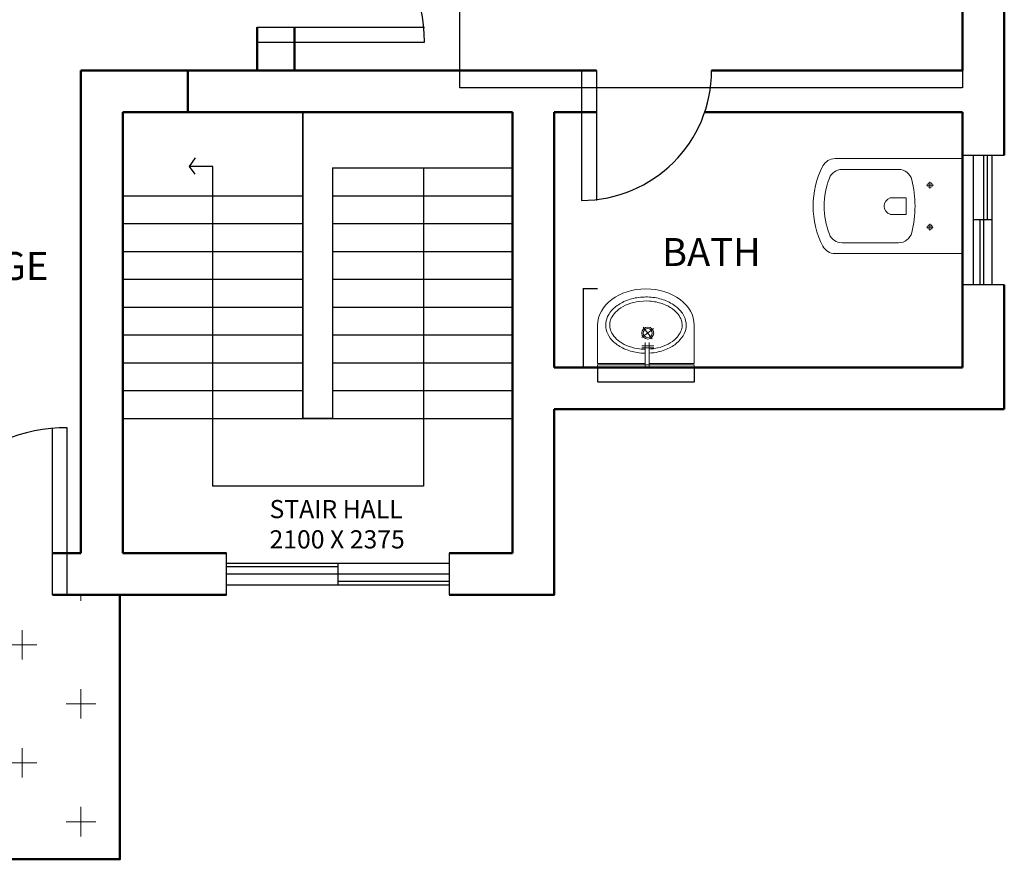
# Model space of a CAD drawing. Units: millimetres. Extents: x -857 to 54106, y -13666 to 13947.
# Tile 21 of 41: x 28540 to 33845, y 3904 to 8428. Entities that reach past the tile are written whole.
import ezdxf

# ---------------------------------------------------------------- set-up
doc = ezdxf.new("R2010")
doc.units = ezdxf.units.MM
for name, color, linetype, lineweight in [('A-ANNO-DIMS', 2, 'Continuous', 18), ('A-AREA-IDEN', 3, 'Continuous', 18), ('A-DOOR', 1, 'Continuous', 25), ('A-FLOR-FIXT', 8, 'Continuous', 18), ('A-FLOR-PATT', 252, 'Continuous', 13), ('A-FLOR-STRS', 30, 'Continuous', 25), ('A-GLAZ', 4, 'Continuous', 25), ('A-SANITARY FITTINGS', 25, 'Continuous', 15), ('A-WALL', 7, 'Continuous', 50)]:
    doc.layers.add(name, color=color, linetype=linetype, lineweight=lineweight)
doc.styles.get("Standard").update_dxf_attribs({"font": 'arial.ttf'})
doc.dimstyles.new('ISO-25', dxfattribs={"dimtxt": 2.5, "dimasz": 2.5, "dimexe": 1.25, "dimexo": 0.625, "dimtad": 1, "dimtxsty": 'Standard', "dimcen": 2.5, "dimadec": 0, "dimazin": 0, "dimtfac": 1, "dimtmove": 0, "dimatfit": 3, "dimfxl": 1, "dimarcsym": 0})

# ---------------------------------------------------------------- blocks, each defined once
blk = doc.blocks.new('A$C0124305E')
at = {"layer": 'A-SANITARY FITTINGS'}
for p, q in [((-8.42, 16.01), (-0.8, 16.01)), ((-0.8, 7.08), (-0.8, 16.01)), ((-7.73, 7.95), (-5.93, 5.62)), ((-4.31, 5.61), (-4.31, 7.96)), ((-3.91, 5.61), (-3.91, 7.96)), ((-5.66, 7.68), (-8, 5.88)), ((0, 7.08), (-4.99, 7.08)), ((0, 6.28), (-4.99, 6.28)), ((-0.8, -3.19), (-0.8, 6.28)), ((-8.42, -3.19), (-0.8, -3.19))]:
    blk.add_line(p, q, dxfattribs=at)
blk.add_lwpolyline([(-0.5, 16.01), (0, 16.01), (0, -3.19), (-0.5, -3.19)], close=True, dxfattribs=at)
for radius in [1.18, 0.885]:
    blk.add_circle((-6.83, 6.78), radius, dxfattribs=at)
at = {"layer": 'A-SANITARY FITTINGS', "extrusion": (0, 0, -1)}
blk.add_ellipse((-8.42, 6.41), major_axis=(0, 9.6), ratio=0.75, start_param=3.141593, end_param=6.283185, dxfattribs=at)
at = {"layer": 'A-SANITARY FITTINGS'}
for points, knots in [([(-2.82, 6.28), (-2.82, 5.74), (-2.87, 5.2), (-3.1, 3.74), (-3.37, 2.86), (-4.09, 1.28), (-4.55, 0.6), (-5.56, -0.5), (-6.12, -0.92), (-7.25, -1.45), (-7.83, -1.58), (-8.98, -1.59), (-9.55, -1.46), (-10.69, -0.93), (-11.25, -0.52), (-12.27, 0.57), (-12.72, 1.25), (-13.45, 2.82), (-13.72, 3.71), (-14.02, 5.56), (-14.05, 6.52), (-13.88, 8.41), (-13.67, 9.32), (-13.04, 10.99), (-12.62, 11.73), (-11.66, 12.96), (-11.12, 13.45), (-10, 14.13), (-9.43, 14.32), (-8.28, 14.45), (-7.7, 14.39), (-6.56, 14), (-5.99, 13.66), (-4.93, 12.71), (-4.44, 12.09), (-3.62, 10.62), (-3.3, 9.78), (-2.96, 8.29), (-2.87, 7.69), (-2.84, 7.08)], [1.58652, 1.58652, 1.58652, 1.58652, 1.780321, 1.780321, 2.120053, 2.120053, 2.459785, 2.459785, 2.799517, 2.799517, 3.139249, 3.139249, 3.478981, 3.478981, 3.818713, 3.818713, 4.158445, 4.158445, 4.498177, 4.498177, 4.837909, 4.837909, 5.177641, 5.177641, 5.517373, 5.517373, 5.857105, 5.857105, 6.196837, 6.196837, 6.536569, 6.536569, 6.876301, 6.876301, 7.216033, 7.216033, 7.555765, 7.555765, 7.774364, 7.774364, 7.774364, 7.774364]), ([(-3.62, 6.29), (-3.62, 5.76), (-3.67, 5.23), (-3.88, 3.96), (-4.1, 3.23), (-4.65, 1.95), (-4.98, 1.39), (-5.72, 0.46), (-6.12, 0.1), (-6.92, -0.44), (-7.32, -0.61), (-8.11, -0.8), (-8.5, -0.81), (-9.28, -0.69), (-9.68, -0.55), (-10.48, -0.08), (-10.89, 0.24), (-11.67, 1.13), (-12.05, 1.7), (-12.66, 3.01), (-12.9, 3.76), (-13.2, 5.38), (-13.25, 6.28), (-13.13, 8.02), (-12.95, 8.88), (-12.42, 10.42), (-12.06, 11.12), (-11.23, 12.25), (-10.77, 12.7), (-9.92, 13.26), (-9.53, 13.43), (-8.78, 13.62), (-8.41, 13.64), (-7.66, 13.54), (-7.28, 13.42), (-6.51, 13.02), (-6.12, 12.73), (-5.35, 11.95), (-4.97, 11.43), (-4.34, 10.23), (-4.08, 9.54), (-3.76, 8.24), (-3.67, 7.64), (-3.63, 7.03)], [1.58652, 1.58652, 1.58652, 1.58652, 1.790653, 1.790653, 2.093007, 2.093007, 2.384527, 2.384527, 2.676047, 2.676047, 2.967567, 2.967567, 3.259087, 3.259087, 3.550608, 3.550608, 3.842128, 3.842128, 4.155456, 4.155456, 4.468784, 4.468784, 4.806699, 4.806699, 5.144614, 5.144614, 5.482529, 5.482529, 5.820444, 5.820444, 6.099515, 6.099515, 6.378586, 6.378586, 6.657656, 6.657656, 6.936727, 6.936727, 7.23864, 7.23864, 7.540552, 7.540552, 7.774364, 7.774364, 7.774364, 7.774364])]:
    blk.add_open_spline(points, degree=3, knots=knots, dxfattribs=at)
blk = doc.blocks.new('A$C7d9d00ca')
at = {"layer": 'A-SANITARY FITTINGS'}
for p, q in [((0, 0), (-13.78, 0)), ((-13.78, -18.49), (-13.78, 0)), ((0, -18.49), (0, 0)), ((-9.94, -4.23), (-9.94, -5.23)), ((-3.84, -4.24), (-3.84, -5.24)), ((-10.42, -4.72), (-9.43, -4.72)), ((-3.36, -4.73), (-4.34, -4.73)), ((-12.2, -9.27), (-12.2, -17.48)), ((-1.57, -9.27), (-1.57, -17.48))]:
    blk.add_line(p, q, dxfattribs=at)
for points in [[(-8.08, -8.19), (-5.7, -8.19), (-5.7, -8.19), (-5.7, -10.48)], [(-8.08, -8.19), (-8.08, -10.48)]]:
    blk.add_lwpolyline(points, dxfattribs=at)
for centre in [(-9.94, -4.72), (-3.84, -4.73)]:
    blk.add_circle(centre, 0.342, dxfattribs=at)
for centre, radius, start, end in [((-6.89, -22.82), 15.93, 76.135, 103.8652), ((-10.24, -9.27), 1.97, 103.8652, 180), ((-3.54, -9.27), 1.97, 0.0003, 76.135), ((-6.89, -10.13), 1.24, 196.5098, 343.4902), ((-11.81, -18.49), 1.97, 180, 242.8074), ((-10.24, -17.48), 1.97, 180, 248.6555), ((-3.54, -17.48), 1.97, 291.3447, 0.0003), ((-1.97, -18.49), 1.97, 297.1926, 0), ((-6.89, -8.92), 11.16, 248.6555, 291.3447), ((-6.89, -8.92), 12.74, 242.8074, 297.1926)]:
    blk.add_arc(centre, radius, start, end, dxfattribs=at)
blk = doc.blocks.new('DOOR-900')
blk.add_line((11417.3, 9811.5), (12317.3, 9811.5))
blk.add_arc((11417.3, 9811.5), 900, 0, 90)
blk = doc.blocks.new('DOOR-700')
blk.add_line((8245.5, 10779.2), (8245.5, 11479.2))
blk.add_arc((8245.5, 10779.2), 700, 90, 180)
blk = doc.blocks.new('WIN-1200')
for p, q in [((9371.3, 11750.2), (10571.3, 11750.2)), ((9371.3, 11731.7), (9971.3, 11731.7)), ((9971.3, 11750.2), (9971.3, 11630.7)), ((9371.3, 11691.7), (10571.3, 11691.7)), ((10571.3, 11630.7), (9371.3, 11630.7)), ((9971.3, 11651.7), (10571.3, 11651.7))]:
    blk.add_line(p, q)
for points in [[(9371.3, 11579.2), (9371.3, 11804.2)], [(10571.3, 11804.2), (10571.3, 11579.2)]]:
    blk.add_lwpolyline(points)
blk = doc.blocks.new('WIN-700')
for p, q in [((3626.3, 8304.2), (3626.3, 9004.2)), ((3679.8, 9004.2), (3679.8, 8304.2)), ((3699.8, 9004.2), (3699.8, 8654.2)), ((3724.4, 9004.2), (3724.4, 8304.2)), ((3724.4, 8654.2), (3626.3, 8654.2)), ((3659.8, 8654.2), (3659.8, 8304.2))]:
    blk.add_line(p, q)
for points in [[(3567.3, 9004.2), (3792.3, 9004.2)], [(3792.3, 8304.2), (3567.3, 8304.2)]]:
    blk.add_lwpolyline(points)
blk = doc.blocks.new('*D41')
at = {"layer": 'A-ANNO-DIMS', "color": 0, "lineweight": -2, "transparency": 16777216}
for p, q in [((31653.8, 6553.6), (31653.8, 6474.9)), ((32174.2, 6553.6), (32174.2, 6474.9)), ((31656.3, 6476.2), (32171.7, 6476.2))]:
    blk.add_line(p, q, dxfattribs=at)
at = {"layer": 'A-ANNO-DIMS', "color": 0, "transparency": 16777216}
for points in [[(31656.3, 6476.6), (31656.3, 6475.8), (31653.8, 6476.2)], [(32171.7, 6476.6), (32171.7, 6475.8), (32174.2, 6476.2)]]:
    blk.add_solid(points, dxfattribs=at)
at = {"layer": 'Defpoints', "color": 0, "transparency": 16777216}
for p in [(31653.8, 6554.2), (32174.2, 6554.2), (32174.2, 6476.2)]:
    blk.add_point(p, dxfattribs=at)
at = {"layer": 'A-ANNO-DIMS', "color": 0, "transparency": 16777216, "insert": (31914, 6478.1), "char_height": 2.5, "attachment_point": 5}
blk.add_mtext('WASH BASIN 520 TYP.', dxfattribs=at)
blk = doc.blocks.new('*D42')
at = {"layer": 'A-ANNO-DIMS', "color": 0, "lineweight": -2, "transparency": 16777216}
for p, q in [((31653.2, 6977.5), (31574.5, 6977.5)), ((31575.8, 6975), (31575.8, 6556.7)), ((31653.2, 6554.2), (31574.5, 6554.2))]:
    blk.add_line(p, q, dxfattribs=at)
at = {"layer": 'A-ANNO-DIMS', "color": 0, "transparency": 16777216}
for points in [[(31575.3, 6975), (31576.2, 6975), (31575.8, 6977.5)], [(31575.3, 6556.7), (31576.2, 6556.7), (31575.8, 6554.2)]]:
    blk.add_solid(points, dxfattribs=at)
at = {"layer": 'Defpoints', "color": 0, "transparency": 16777216}
for p in [(31653.8, 6977.5), (31575.8, 6554.2), (31653.8, 6554.2)]:
    blk.add_point(p, dxfattribs=at)
at = {"layer": 'A-ANNO-DIMS', "color": 0, "transparency": 16777216, "insert": (31573.9, 6765.8), "char_height": 2.5, "attachment_point": 5, "rotation": 90}
blk.add_mtext('423 TYP.', dxfattribs=at)
blk = doc.blocks.new('*D47')
at = {"layer": 'A-ANNO-DIMS', "color": 0, "lineweight": -2, "transparency": 16777216}
for p, q in [((30909.3, 8468.4), (30909.3, 8061.1)), ((33620.1, 8468.4), (33620.1, 8061.1)), ((30911.8, 8062.4), (33617.6, 8062.4))]:
    blk.add_line(p, q, dxfattribs=at)
at = {"layer": 'A-ANNO-DIMS', "color": 0, "transparency": 16777216}
for points in [[(30911.8, 8062.8), (30911.8, 8062), (30909.3, 8062.4)], [(33617.6, 8062.8), (33617.6, 8062), (33620.1, 8062.4)]]:
    blk.add_solid(points, dxfattribs=at)
at = {"layer": 'Defpoints', "color": 0, "transparency": 16777216}
for p in [(30909.3, 8469), (33620.1, 8469), (33620.1, 8062.4)]:
    blk.add_point(p, dxfattribs=at)
at = {"layer": 'A-ANNO-DIMS', "color": 0, "transparency": 16777216, "insert": (32264.7, 8064.3), "char_height": 2.5, "attachment_point": 5}
blk.add_mtext('ROUND BED 2711 TYP.', dxfattribs=at)

msp = doc.modelspace()

# ---------------------------------------------------------------- hatches: boundary and pattern name
at = {"layer": 'A-FLOR-PATT'}
h = msp.add_hatch(dxfattribs=at)
h.set_pattern_fill('CROSS', color=256, scale=50)
h.set_pattern_definition([(0, (11962.88, -2561.3), (317.5, 317.5), [158.75, -476.25]), (90, (12042.26, -2640.7), (-317.5, 317.5), [158.75, -476.25])])
h.paths.add_polyline_path([(29079.919, 5329.231), (28716.385, 5329.231), (27076.385, 5329.231), (26996.385, 5329.231), (26539.053, 5329.231), (26539.053, 5380.706), (25339.053, 5380.706), (25339.053, 5329.231), (24870.079, 5329.231), (24870.079, 3903.799), (29079.919, 3903.799)])

# ---------------------------------------------------------------- linework, layer by layer
at = {"layer": 'A-DOOR'}
for p, q in [((29820.079, 8387.298), (30720.079, 8387.298)), ((31647.549, 8154.231), (31647.549, 7454.231)), ((28716.385, 5329.231), (28716.385, 6229.231)), ((28796.385, 5329.231), (28716.385, 5329.231))]:
    msp.add_line(p, q, dxfattribs=at)
at = {"layer": 'A-FLOR-STRS'}
for p, q in [((29445.079, 7929.231), (29095.079, 7929.231)), ((30065.079, 7929.231), (30065.079, 6279.231)), ((30225.079, 7629.231), (31195.079, 7629.231)), ((30225.079, 7629.231), (30225.079, 6279.231)), ((29095.079, 7479.231), (30065.079, 7479.231)), ((30225.079, 7479.231), (31195.079, 7479.231)), ((29095.079, 7329.231), (30065.079, 7329.231)), ((30225.079, 7329.231), (31195.079, 7329.231)), ((29095.079, 7179.231), (30065.079, 7179.231)), ((30225.079, 7179.231), (31195.079, 7179.231)), ((29095.079, 7029.231), (30065.079, 7029.231)), ((30225.079, 7029.231), (31195.079, 7029.231)), ((29095.079, 6879.231), (30065.079, 6879.231)), ((30225.079, 6879.231), (31195.079, 6879.231)), ((29095.079, 6729.231), (30065.079, 6729.231)), ((30225.079, 6729.231), (31195.079, 6729.231)), ((29095.079, 6579.231), (30065.079, 6579.231)), ((30225.079, 6579.231), (31195.079, 6579.231)), ((29095.079, 6429.231), (30065.079, 6429.231)), ((30225.079, 6429.231), (31195.079, 6429.231)), ((29095.079, 6279.231), (31195.079, 6279.231))]:
    msp.add_line(p, q, dxfattribs=at)
for points in [[(30225.079, 7629.231), (30225.079, 6279.231), (30065.079, 6279.231), (30065.079, 7929.231), (30225.079, 7929.231)], [(29484.771, 7684.139), (29453.317, 7637.854), (29483.619, 7594.913)], [(30716.035, 7629.231), (30716.035, 5914.255), (29580.079, 5914.255), (29580.079, 7637.854), (29453.317, 7637.854)]]:
    msp.add_lwpolyline(points, dxfattribs=at)
at = {"layer": 'A-WALL'}
for p, q in [((33620.079, 11404.231), (33620.079, 8154.231)), ((33845.069, 9314.82), (33845.063, 8154.231)), ((29820.079, 8154.231), (29820.079, 8387.298)), ((30020.079, 8387.298), (30020.079, 8154.231)), ((28870.079, 5554.231), (28870.079, 8154.231)), ((29095.079, 8154.231), (28870.079, 8154.231)), ((29095.079, 8154.231), (29445.079, 8154.231)), ((29445.079, 8154.231), (29445.079, 7929.231)), ((29445.079, 8154.231), (30845.079, 8154.231)), ((31647.549, 8154.231), (29820.079, 8154.231)), ((30845.079, 8154.231), (31195.079, 8154.231)), ((31195.079, 8154.231), (31647.549, 8154.231)), ((33620.079, 8154.231), (32267.549, 8154.231)), ((32267.549, 8154.231), (33620.079, 8154.231)), ((33845.063, 8154.231), (33845.063, 7698.848)), ((29095.079, 5554.231), (29095.079, 7929.231)), ((29095.079, 7929.231), (30845.079, 7929.231)), ((29445.079, 7929.231), (30845.079, 7929.231)), ((30845.079, 7929.231), (31195.079, 7929.231)), ((31195.079, 7929.231), (31195.079, 5554.231)), ((31420.079, 7929.231), (31420.079, 6554.231)), ((31647.549, 7929.231), (31420.079, 7929.231)), ((33620.079, 7929.231), (32230.403, 7929.231)), ((33620.079, 6554.231), (33620.079, 7929.231)), ((33845.063, 6998.848), (33845.063, 6329.231)), ((31420.079, 6554.231), (33620.079, 6554.231)), ((31420.079, 6329.231), (33845.063, 6329.231)), ((28796.385, 5554.231), (28716.385, 5554.231)), ((28870.079, 5554.231), (28796.385, 5554.231)), ((29653.592, 5554.231), (29095.079, 5554.231)), ((29653.592, 5554.231), (29095.079, 5554.231)), ((31195.079, 5554.231), (30853.592, 5554.231)), ((31195.079, 5554.231), (30853.592, 5554.231))]:
    msp.add_line(p, q, dxfattribs=at)
for points in [[(31420.079, 7929.231), (31420.079, 6554.231)], [(31420.079, 6329.231), (31420.079, 5329.231), (30853.592, 5329.231)], [(25339.053, 5329.231), (24870.079, 5329.231), (24870.079, 3903.799), (29079.919, 3903.799), (29079.919, 5329.231), (28716.385, 5329.231)], [(29653.592, 5329.231), (28716.385, 5329.231)]]:
    msp.add_lwpolyline(points, dxfattribs=at)

# ---------------------------------------------------------------- block references
at = {"layer": 'A-DOOR'}
msp.add_blockref('DOOR-900', (18402.799, -1504.183), dxfattribs=at)
for name, p, rotation in [('DOOR-700', (39813.095, 18933.462), 180), ('DOOR-900', (38607.866, -6088.049), 89.99999999999991)]:
    msp.add_blockref(name, p, dxfattribs=dict(at, rotation=rotation))
at = {"layer": 'A-FLOR-FIXT'}
for name, p, xscale, yscale, zscale, rotation in [('A$C7d9d00ca', (33620.079, 7167.496), 37.15841229138232, 37.15841229138232, 37.15841229138232, 270), ('A$C0124305E', (31740.18, 6554.231), 27.10344997005861, 27.10344997005861, 27.10344997005861, 270.0000000004072)]:
    msp.add_blockref(name, p, dxfattribs=dict(at, xscale=xscale, yscale=yscale, zscale=zscale, rotation=rotation))
at = {"layer": 'A-GLAZ'}
for name, p in [('WIN-700', (30052.799, -1305.383)), ('WIN-1200', (20282.252, -6250))]:
    msp.add_blockref(name, p, dxfattribs=at)

# ---------------------------------------------------------------- texts
at = {"layer": 'A-AREA-IDEN', "attachment_point": 1}
for s, insert, char_height in [('\\pxt0;BATH', (32000.685, 7251.442), 150.4846), ('\\pxt0;PASSAGE', (27807.484, 7176.075), 150.48461), ('\\pxt0;STAIR HALL\\P2100 X 2375', (29885.918, 5839.865), 97.80511)]:
    msp.add_mtext_dynamic_manual_height_columns(s, width=2554.22693, gutter_width=18810.576, heights=[2595.835], dxfattribs=dict(at, insert=insert, char_height=char_height))

# ---------------------------------------------------------------- dimensions: what is measured, and where the dimension line sits
at = {"layer": 'A-ANNO-DIMS'}
dim = msp.add_linear_dim(base=(33620.079, 8062.375), p1=(30909.254, 8468.999), p2=(33620.079, 8468.999), text='ROUND BED <> TYP.', dimstyle='ISO-25', override={"dimdec": 0, "dimrnd": 0, "dimzin": 0, "dimlunit": 2}, dxfattribs=at)
dim.commit()
dim.dimension.update_dxf_attribs({"geometry": '*D47', "text_midpoint": (32264.666, 8064.293)})
for base, p1, p2, angle, text, picture, middle in [((31575.763, 6554.231), (31653.821, 6977.459), (31653.821, 6554.231), 270, '<> TYP.', '*D42', (31573.861, 6765.845)), ((32174.207, 6476.173), (31653.821, 6554.231), (32174.207, 6554.231), 0, 'WASH BASIN <> TYP.', '*D41', (31914.014, 6478.091))]:
    dim = msp.add_linear_dim(base=base, p1=p1, p2=p2, angle=angle, text=text, dimstyle='ISO-25', override={"dimdec": 0, "dimrnd": 0, "dimzin": 0, "dimlunit": 2}, dxfattribs=at)
    dim.commit()
    dim.dimension.update_dxf_attribs({"geometry": picture, "text_midpoint": middle})

doc.saveas('drawing.dxf')
